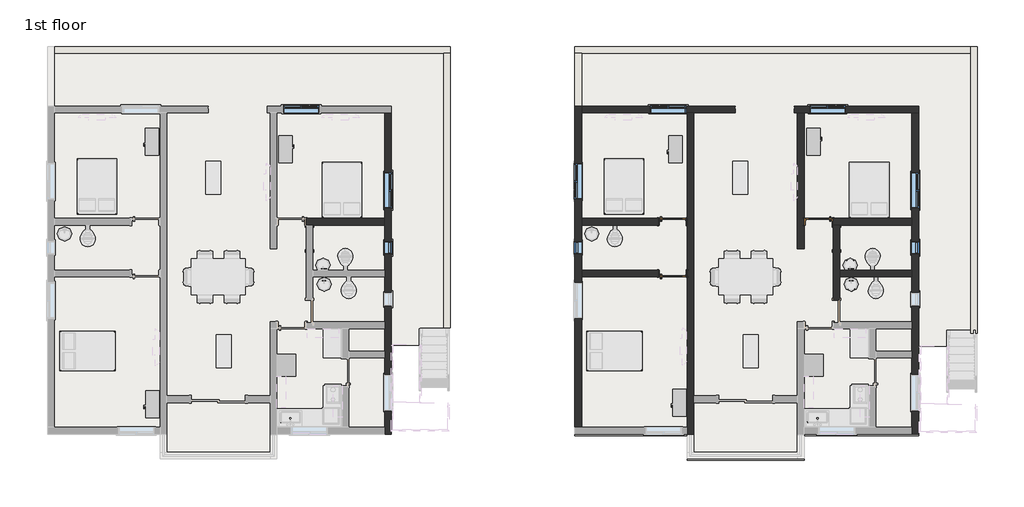
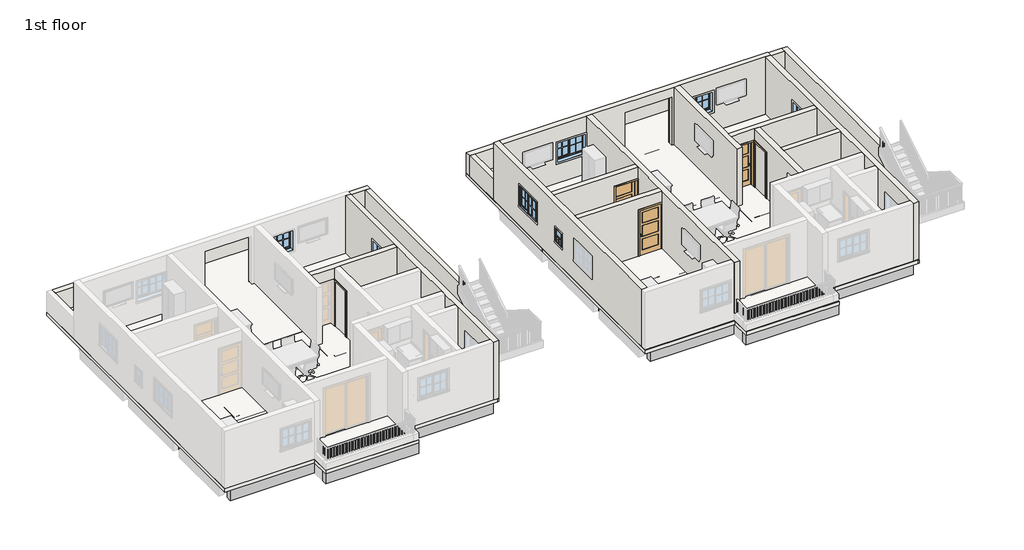
# One storey, part 2 of 8: 18 walls, 14 beams, 9 windows, 5 doors, 2 slabs.
"""IFC4 building model written with IfcOpenShell, lengths in millimetres."""

from ifc_helpers import new_model, si_unit, frame, origin, place, context, project, spatial, polyline, outline, extrude, faceted_brep, transform, mapped, element, save
from components import door_2334f446, door_80766924, door_85036156, window_608ea798, window_2eef0573, window_a5b1ea32

model = new_model("IFC4")

# Units and contexts
model_context = context("Model", 3, world=origin())
ifc_project = project(units=[si_unit("LENGTHUNIT", "METRE", prefix="MILLI")], contexts=[model_context])

# Site, building, storey
site = spatial("IfcSite", under=ifc_project)
building = spatial("IfcBuilding", under=site)
storey = spatial("IfcBuildingStorey", under=building, Name="1st floor", Elevation=3810.0)

# Beams
placement = place(None, origin())
element("IfcBeam", 1, ObjectType="Concrete-Rectangular Beam", at=placement, inside=storey, context=model_context, shape_type="SweptSolid", body=[
    extrude(outline(polyline([(-16071.9993763, -4605.3064015), (-16071.9993763, -4376.7064015), (-12490.5993763, -4376.7064015), (-12490.5993763, -4605.3064015), (-16071.9993763, -4605.3064015)])), frame((0.0, 0.0, 3200.4), z_axis=(0.0, 0.0, 1.0), x_axis=(1.0, 0.0, 0.0)), (0.0, 0.0, 1.0), 609.6),
])
element("IfcBeam", 2, ObjectType="Concrete-Rectangular Beam", at=placement, inside=storey, context=model_context, shape_type="Brep", body=[
    faceted_brep([(-8528.1993763, -5443.5064015, 3810.0), (-8528.1993763, -5214.9064015, 3810.0), (-8756.7993763, -5214.9064015, 3810.0), (-12261.9993763, -5214.9064015, 3810.0), (-12490.5993763, -5214.9064015, 3810.0), (-12490.5993763, -5443.5064015, 3810.0), (-8528.1993763, -5443.5064015, 3200.4), (-12490.5993763, -5443.5064015, 3200.4), (-8528.1993763, -5214.9064015, 3200.4), (-12490.5993763, -5214.9064015, 3200.4), (-12261.9993763, -5214.9064015, 3200.4), (-8756.7993763, -5214.9064015, 3200.4)], [[[0, 1, 2, 3, 4, 5]], [[6, 0, 5, 7]], [[8, 6, 7, 9, 10, 11]], [[1, 8, 11, 10, 9, 4, 3, 2]], [[1, 0, 6, 8]], [[5, 4, 9, 7]]]),
])
element("IfcBeam", 3, ObjectType="Concrete-Rectangular Beam", at=placement, inside=storey, context=model_context, shape_type="Brep", body=[
    faceted_brep([(-8528.1993763, -4376.7064015, 3810.0), (-8528.1993763, -4605.3064015, 3810.0), (-4870.5993763, -4605.3064015, 3810.0), (-4870.5993763, -4376.7064015, 3810.0), (-6089.7993763, -4376.7064015, 3810.0), (-6318.3993763, -4376.7064015, 3810.0), (-8528.1993763, -4376.7064015, 3200.4), (-4870.5993763, -4376.7064015, 3200.4), (-6089.7993763, -4376.7064015, 3200.4), (-6318.3993763, -4376.7064015, 3200.4), (-8528.1993763, -4605.3064015, 3200.4), (-4870.5993763, -4605.3064015, 3200.4)], [[[0, 1, 2, 3, 4, 5]], [[6, 0, 5, 4, 3, 7, 8, 9]], [[10, 6, 9, 8, 7, 11]], [[1, 10, 11, 2]], [[1, 0, 6, 10]], [[3, 2, 11, 7]]]),
])
element("IfcBeam", 4, ObjectType="Concrete-Rectangular Beam", at=placement, inside=storey, context=model_context, shape_type="Brep", body=[
    faceted_brep([(-8528.1993763, -795.3064015, 3810.0), (-8528.1993763, -1023.9064015, 3810.0), (-6318.3993763, -1023.9064015, 3810.0), (-6089.7993763, -1023.9064015, 3810.0), (-4870.5993763, -1023.9064015, 3810.0), (-4870.5993763, -795.3064015, 3810.0), (-7308.9993763, -795.3064015, 3810.0), (-7537.5993763, -795.3064015, 3810.0), (-8528.1993763, -795.3064015, 3200.4), (-4870.5993763, -795.3064015, 3200.4), (-7308.9993763, -795.3064015, 3200.4), (-7537.5993763, -795.3064015, 3200.4), (-8528.1993763, -1023.9064015, 3200.4), (-4870.5993763, -1023.9064015, 3200.4), (-6089.7993763, -1023.9064015, 3200.4), (-6318.3993763, -1023.9064015, 3200.4)], [[[0, 1, 2, 3, 4, 5, 6, 7]], [[8, 0, 7, 6, 5, 9, 10, 11]], [[12, 8, 11, 10, 9, 13, 14, 15]], [[1, 12, 15, 14, 13, 4, 3, 2]], [[1, 0, 8, 12]], [[5, 4, 13, 9]]]),
])
element("IfcBeam", 5, ObjectType="Concrete-Rectangular Beam", at=placement, inside=storey, context=model_context, shape_type="Brep", body=[
    faceted_brep([(-6318.3993763, -4376.7064015, 3810.0), (-6089.7993763, -4376.7064015, 3810.0), (-6089.7993763, -2014.5064015, 3810.0), (-6089.7993763, -1785.9064015, 3810.0), (-6089.7993763, -1023.9064015, 3810.0), (-6318.3993763, -1023.9064015, 3810.0), (-6089.7993763, -4376.7064015, 3200.4), (-6089.7993763, -2014.5064015, 3200.4), (-6089.7993763, -1785.9064015, 3200.4), (-6089.7993763, -1023.9064015, 3200.4), (-6318.3993763, -4376.7064015, 3200.4), (-6318.3993763, -1023.9064015, 3200.4)], [[[0, 1, 2, 3, 4, 5]], [[1, 6, 7, 8, 9, 4, 3, 2]], [[6, 10, 11, 9, 8, 7]], [[10, 0, 5, 11]], [[1, 0, 10, 6]], [[5, 4, 9, 11]]]),
])
element("IfcBeam", 6, ObjectType="Concrete-Rectangular Beam", at=placement, inside=storey, context=model_context, shape_type="SweptSolid", body=[
    extrude(outline(polyline([(-4870.5993763, -1785.9064015), (-4870.5993763, -2014.5064015), (-6089.7993763, -2014.5064015), (-6089.7993763, -1785.9064015), (-4870.5993763, -1785.9064015)])), frame((0.0, 0.0, 3200.4), z_axis=(0.0, 0.0, 1.0), x_axis=(1.0, 0.0, 0.0)), (0.0, 0.0, 1.0), 609.6),
])
element("IfcBeam", 7, ObjectType="Concrete-Rectangular Beam", at=placement, inside=storey, context=model_context, shape_type="Brep", body=[
    faceted_brep([(-8756.7993763, -1023.9064015, 3810.0), (-8756.7993763, -795.3064015, 3810.0), (-12261.9993763, -795.3064015, 3810.0), (-12261.9993763, -1023.9064015, 3810.0), (-8756.7993763, -795.3064015, 3200.4), (-12261.9993763, -795.3064015, 3200.4), (-8756.7993763, -1023.9064015, 3200.4), (-12261.9993763, -1023.9064015, 3200.4)], [[[0, 1, 2, 3]], [[1, 4, 5, 2]], [[4, 6, 7, 5]], [[6, 0, 3, 7]], [[1, 0, 6, 4]], [[3, 2, 5, 7]]]),
    faceted_brep([(-16071.9993763, -1023.9064015, 3810.0), (-16071.9993763, -795.3064015, 3810.0), (-16071.9993763, -795.3064015, 3200.4), (-16071.9993763, -1023.9064015, 3200.4), (-12490.5993763, -795.3064015, 3810.0), (-12490.5993763, -1023.9064015, 3810.0), (-12490.5993763, -1023.9064015, 3200.4), (-12490.5993763, -795.3064015, 3200.4), (-13481.1993763, -795.3064015, 3810.0), (-13709.7993763, -795.3064015, 3810.0), (-13481.1993763, -795.3064015, 3200.4), (-13709.7993763, -795.3064015, 3200.4)], [[[0, 1, 2, 3]], [[4, 5, 6, 7]], [[1, 0, 5, 4, 8, 9]], [[2, 1, 9, 8, 4, 7, 10, 11]], [[3, 2, 11, 10, 7, 6]], [[0, 3, 6, 5]]]),
])
element("IfcBeam", 8, ObjectType="Concrete-Rectangular Beam", at=placement, inside=storey, context=model_context, shape_type="SweptSolid", body=[
    extrude(outline(polyline([(-12261.9993763, -3538.5064015), (-12261.9993763, -3309.9064015), (-8756.7993763, -3309.9064015), (-8756.7993763, -3538.5064015), (-12261.9993763, -3538.5064015)])), frame((0.0, 0.0, 3200.4), z_axis=(0.0, 0.0, 1.0), x_axis=(1.0, 0.0, 0.0)), (0.0, 0.0, 1.0), 609.6),
])
element("IfcBeam", 9, ObjectType="Concrete-Rectangular Beam", at=placement, inside=storey, context=model_context, shape_type="SweptSolid", body=[
    extrude(outline(polyline([(1802.5761273, -4605.3064015), (1802.5761273, -4376.7064015), (5383.9761273, -4376.7064015), (5383.9761273, -4605.3064015), (1802.5761273, -4605.3064015)])), frame((0.0, 0.0, 3200.4), z_axis=(0.0, 0.0, 1.0), x_axis=(1.0, 0.0, 0.0)), (0.0, 0.0, 1.0), 609.6),
])
element("IfcBeam", 10, ObjectType="Concrete-Rectangular Beam", at=placement, inside=storey, context=model_context, shape_type="Brep", body=[
    faceted_brep([(9346.3761273, -5443.5064015, 3810.0), (9346.3761273, -5214.9064015, 3810.0), (9117.7761273, -5214.9064015, 3810.0), (5612.5761273, -5214.9064015, 3810.0), (5383.9761273, -5214.9064015, 3810.0), (5383.9761273, -5443.5064015, 3810.0), (9346.3761273, -5443.5064015, 3200.4), (5383.9761273, -5443.5064015, 3200.4), (9346.3761273, -5214.9064015, 3200.4), (5383.9761273, -5214.9064015, 3200.4), (5612.5761273, -5214.9064015, 3200.4), (9117.7761273, -5214.9064015, 3200.4)], [[[0, 1, 2, 3, 4, 5]], [[6, 0, 5, 7]], [[8, 6, 7, 9, 10, 11]], [[1, 8, 11, 10, 9, 4, 3, 2]], [[1, 0, 6, 8]], [[5, 4, 9, 7]]]),
])
element("IfcBeam", 11, ObjectType="Concrete-Rectangular Beam", at=placement, inside=storey, context=model_context, shape_type="Brep", body=[
    faceted_brep([(9346.3761273, -4376.7064015, 3810.0), (9346.3761273, -4605.3064015, 3810.0), (13003.9761273, -4605.3064015, 3810.0), (13003.9761273, -4376.7064015, 3810.0), (11784.7761273, -4376.7064015, 3810.0), (11556.1761273, -4376.7064015, 3810.0), (9346.3761273, -4376.7064015, 3200.4), (13003.9761273, -4376.7064015, 3200.4), (11784.7761273, -4376.7064015, 3200.4), (11556.1761273, -4376.7064015, 3200.4), (9346.3761273, -4605.3064015, 3200.4), (13003.9761273, -4605.3064015, 3200.4)], [[[0, 1, 2, 3, 4, 5]], [[6, 0, 5, 4, 3, 7, 8, 9]], [[10, 6, 9, 8, 7, 11]], [[1, 10, 11, 2]], [[1, 0, 6, 10]], [[3, 2, 11, 7]]]),
])
element("IfcBeam", 12, ObjectType="Concrete-Rectangular Beam", at=placement, inside=storey, context=model_context, shape_type="Brep", body=[
    faceted_brep([(11556.1761273, -4376.7064015, 3810.0), (11784.7761273, -4376.7064015, 3810.0), (11784.7761273, -2014.5064015, 3810.0), (11784.7761273, -1785.9064015, 3810.0), (11784.7761273, -1023.9064015, 3810.0), (11556.1761273, -1023.9064015, 3810.0), (11784.7761273, -4376.7064015, 3200.4), (11784.7761273, -2014.5064015, 3200.4), (11784.7761273, -1785.9064015, 3200.4), (11784.7761273, -1023.9064015, 3200.4), (11556.1761273, -4376.7064015, 3200.4), (11556.1761273, -1023.9064015, 3200.4)], [[[0, 1, 2, 3, 4, 5]], [[1, 6, 7, 8, 9, 4, 3, 2]], [[6, 10, 11, 9, 8, 7]], [[10, 0, 5, 11]], [[1, 0, 10, 6]], [[5, 4, 9, 11]]]),
])
element("IfcBeam", 13, ObjectType="Concrete-Rectangular Beam", at=placement, inside=storey, context=model_context, shape_type="Brep", body=[
    faceted_brep([(9117.7761273, -1023.9064015, 3810.0), (9117.7761273, -795.3064015, 3810.0), (5612.5761273, -795.3064015, 3810.0), (5612.5761273, -1023.9064015, 3810.0), (9117.7761273, -795.3064015, 3200.4), (5612.5761273, -795.3064015, 3200.4), (9117.7761273, -1023.9064015, 3200.4), (5612.5761273, -1023.9064015, 3200.4)], [[[0, 1, 2, 3]], [[1, 4, 5, 2]], [[4, 6, 7, 5]], [[6, 0, 3, 7]], [[1, 0, 6, 4]], [[3, 2, 5, 7]]]),
    faceted_brep([(1802.5761273, -1023.9064015, 3810.0), (1802.5761273, -795.3064015, 3810.0), (1802.5761273, -795.3064015, 3200.4), (1802.5761273, -1023.9064015, 3200.4), (5383.9761273, -795.3064015, 3810.0), (5383.9761273, -1023.9064015, 3810.0), (5383.9761273, -1023.9064015, 3200.4), (5383.9761273, -795.3064015, 3200.4), (4393.3761273, -795.3064015, 3810.0), (4164.7761273, -795.3064015, 3810.0), (4393.3761273, -795.3064015, 3200.4), (4164.7761273, -795.3064015, 3200.4)], [[[0, 1, 2, 3]], [[4, 5, 6, 7]], [[1, 0, 5, 4, 8, 9]], [[2, 1, 9, 8, 4, 7, 10, 11]], [[3, 2, 11, 10, 7, 6]], [[0, 3, 6, 5]]]),
])
element("IfcBeam", 14, ObjectType="Concrete-Rectangular Beam", at=placement, inside=storey, context=model_context, shape_type="SweptSolid", body=[
    extrude(outline(polyline([(5612.5761273, -3538.5064015), (5612.5761273, -3309.9064015), (9117.7761273, -3309.9064015), (9117.7761273, -3538.5064015), (5612.5761273, -3538.5064015)])), frame((0.0, 0.0, 3200.4), z_axis=(0.0, 0.0, 1.0), x_axis=(1.0, 0.0, 0.0)), (0.0, 0.0, 1.0), 609.6),
])

# Doors
door_shape = door_2334f446(model_context)
element("IfcDoor", 15, ObjectType="Door-Interior-Single-3_Panel_Vert-Wood : 36\" x 80\"", at=placement, inside=storey, context=model_context, shape_type="MappedRepresentation", body=[
    mapped(door_shape, transform((4888.6761273, 2598.7685985, 3810.0), x_axis=(1.0, 0.0, 0.0), y_axis=(0.0, 1.0, 0.0), z_axis=(0.0, 0.0, 1.0))),
])
door_2_shape = door_80766924(model_context)
element("IfcDoor", 16, ObjectType="Door-Interior-Single-3_Panel_Vert-Wood : 36\" x 80\"", at=placement, inside=storey, context=model_context, shape_type="MappedRepresentation", body=[
    mapped(door_2_shape, transform((4888.6761273, 839.8185985, 3810.0), x_axis=(1.0, 0.0, 0.0), y_axis=(0.0, 1.0, 0.0), z_axis=(0.0, 0.0, 1.0))),
])
element("IfcDoor", 17, ObjectType="Door-Interior-Single-3_Panel_Vert-Wood : 36\" x 80\"", at=placement, inside=storey, context=model_context, shape_type="MappedRepresentation", body=[
    mapped(door_2_shape, transform((9841.6761273, 2598.7685985, 3810.0), x_axis=(-1.0, 0.0, 0.0), y_axis=(0.0, -1.0, 0.0), z_axis=(0.0, 0.0, 1.0))),
])
door_3_shape = door_85036156(model_context)
element("IfcDoor", 18, ObjectType="Single-Flush : 30\" x 80\"", at=placement, inside=storey, context=model_context, shape_type="MappedRepresentation", body=[
    mapped(door_3_shape, transform((-7423.2993763, 2024.0935985, 3810.0), x_axis=(0.0, 1.0, 0.0), y_axis=(-1.0, 0.0, 0.0), z_axis=(0.0, 0.0, 1.0))),
])
element("IfcDoor", 19, ObjectType="Single-Flush : 30\" x 80\"", at=placement, inside=storey, context=model_context, shape_type="MappedRepresentation", body=[
    mapped(door_3_shape, transform((10451.2761273, 2024.0935985, 3810.0), x_axis=(0.0, 1.0, 0.0), y_axis=(-1.0, 0.0, 0.0), z_axis=(0.0, 0.0, 1.0))),
])

# Slabs
element("IfcSlab", 20, at=placement, inside=storey, context=model_context, shape_type="SweptSolid", body=[
    extrude(outline(polyline([(-2647.3594779, 8539.1935985), (-2647.3594779, -998.5064015), (-3676.7993763, -998.5064015), (-3676.7993763, -1582.7064015), (-4641.9993763, -1582.7064015), (-4641.9993763, -4605.3064015), (-4692.7993763, -4605.3064015), (-8528.1993763, -4605.3064015), (-8528.1993763, -5443.5064015), (-12490.5993763, -5443.5064015), (-12490.5993763, -4611.6564015), (-16300.5993763, -4611.6564015), (-16300.5993763, 8539.1935985), (-2647.3594779, 8539.1935985)])), frame((0.0, 0.0, 3657.6), z_axis=(0.0, 0.0, 1.0), x_axis=(1.0, 0.0, 0.0)), (0.0, 0.0, 1.0), 152.4),
])
element("IfcSlab", 21, at=placement, inside=storey, context=model_context, shape_type="SweptSolid", body=[
    extrude(outline(polyline([(15227.2160257, 8539.1935985), (15227.2160257, -1093.7564015), (14197.7761273, -1093.7564015), (14197.7761273, -1627.1564015), (13232.5761273, -1627.1564015), (13232.5761273, -4649.7564015), (13181.7761273, -4649.7564015), (9346.3761273, -4649.7564015), (9346.3761273, -5487.9564015), (5383.9761273, -5487.9564015), (5383.9761273, -4656.1064015), (1573.9761273, -4656.1064015), (1573.9761273, 8539.1935985), (15227.2160257, 8539.1935985)])), frame((0.0, 0.0, 3657.6), z_axis=(0.0, 0.0, 1.0), x_axis=(1.0, 0.0, 0.0)), (0.0, 0.0, 1.0), 152.4),
])

# Walls
element("IfcWall", 22, at=placement, inside=storey, context=model_context, shape_type="Brep", body=[
    faceted_brep([(-4870.5993763, 6291.2935985, 3810.0), (-4870.5993763, 2709.8935985, 3810.0), (-4870.5993763, 2481.2935985, 3810.0), (-4870.5993763, 957.2935985, 3810.0), (-4870.5993763, 728.6935985, 3810.0), (-4870.5993763, -795.3064015, 3810.0), (-4870.5993763, -1023.9064015, 3810.0), (-4870.5993763, -1785.9064015, 3810.0), (-4870.5993763, -2014.5064015, 3810.0), (-4870.5993763, -4376.7064015, 3810.0), (-4870.5993763, -4605.3064015, 3810.0), (-4870.5993763, -4605.3064015, 6400.8), (-4870.5993763, -4376.7064015, 6400.8), (-4870.5993763, -2014.5064015, 6400.8), (-4870.5993763, -1785.9064015, 6400.8), (-4870.5993763, -1023.9064015, 6400.8), (-4870.5993763, -795.3064015, 6400.8), (-4870.5993763, 728.6935985, 6400.8), (-4870.5993763, 957.2935985, 6400.8), (-4870.5993763, 2481.2935985, 6400.8), (-4870.5993763, 2709.8935985, 6400.8), (-4870.5993763, 6291.2935985, 6400.8), (-4870.5993763, 4271.9935985, 5638.8), (-4870.5993763, 3052.7935985, 5638.8), (-4870.5993763, 3052.7935985, 4724.4), (-4870.5993763, 4271.9935985, 4724.4), (-4870.5993763, -249.2064015, 5334.0), (-4870.5993763, -249.2064015, 4724.4), (-4870.5993763, 182.5935985, 4724.4), (-4870.5993763, 182.5935985, 5334.0), (-4870.5993763, 1503.3935985, 5334.0), (-4870.5993763, 1503.3935985, 4724.4), (-4870.5993763, 1935.1935985, 4724.4), (-4870.5993763, 1935.1935985, 5334.0), (-4870.5993763, -3805.2064015, 5638.8), (-4870.5993763, -3805.2064015, 4724.4), (-4870.5993763, -2586.0064015, 4724.4), (-4870.5993763, -2586.0064015, 5638.8), (-4641.9993763, 6291.2935985, 3810.0), (-4641.9993763, 6291.2935985, 6400.8), (-4641.9993763, -4605.3064015, 6400.8), (-4641.9993763, -4605.3064015, 3810.0), (-4641.9993763, 4271.9935985, 5638.8), (-4641.9993763, 4271.9935985, 4724.4), (-4641.9993763, 3052.7935985, 4724.4), (-4641.9993763, 3052.7935985, 5638.8), (-4641.9993763, -249.2064015, 5334.0), (-4641.9993763, 182.5935985, 5334.0), (-4641.9993763, 182.5935985, 4724.4), (-4641.9993763, -249.2064015, 4724.4), (-4641.9993763, 1503.3935985, 5334.0), (-4641.9993763, 1935.1935985, 5334.0), (-4641.9993763, 1935.1935985, 4724.4), (-4641.9993763, 1503.3935985, 4724.4), (-4641.9993763, -3805.2064015, 5638.8), (-4641.9993763, -2586.0064015, 5638.8), (-4641.9993763, -2586.0064015, 4724.4), (-4641.9993763, -3805.2064015, 4724.4)], [[[0, 1, 2, 3, 4, 5, 6, 7, 8, 9, 10, 11, 12, 13, 14, 15, 16, 17, 18, 19, 20, 21], [22, 23, 24, 25], [26, 27, 28, 29], [30, 31, 32, 33], [34, 35, 36, 37]], [[38, 39, 40, 41], [42, 43, 44, 45], [46, 47, 48, 49], [50, 51, 52, 53], [54, 55, 56, 57]], [[10, 9, 8, 7, 6, 5, 4, 3, 2, 1, 0, 38, 41]], [[21, 20, 19, 18, 17, 16, 15, 14, 13, 12, 11, 40, 39]], [[0, 21, 39, 38]], [[11, 10, 41, 40]], [[43, 42, 22, 25]], [[44, 43, 25, 24]], [[45, 44, 24, 23]], [[42, 45, 23, 22]], [[27, 26, 46, 49]], [[28, 27, 49, 48]], [[29, 28, 48, 47]], [[26, 29, 47, 46]], [[31, 30, 50, 53]], [[32, 31, 53, 52]], [[33, 32, 52, 51]], [[30, 33, 51, 50]], [[35, 34, 54, 57]], [[36, 35, 57, 56]], [[37, 36, 56, 55]], [[34, 37, 55, 54]]]),
])
element("IfcWall", 23, at=placement, inside=storey, context=model_context, shape_type="Brep", body=[
    faceted_brep([(-4870.5993763, 2481.2935985, 6400.8), (-7308.9993763, 2481.2935985, 6400.8), (-7537.5993763, 2481.2935985, 6400.8), (-8528.1993763, 2481.2935985, 6400.8), (-8528.1993763, 2481.2935985, 3810.0), (-8515.4993763, 2481.2935985, 3810.0), (-8515.4993763, 2481.2935985, 5867.4), (-7550.2993763, 2481.2935985, 5867.4), (-7550.2993763, 2481.2935985, 3810.0), (-7537.5993763, 2481.2935985, 3810.0), (-7308.9993763, 2481.2935985, 3810.0), (-4870.5993763, 2481.2935985, 3810.0), (-8528.1993763, 2709.8935985, 6400.8), (-4870.5993763, 2709.8935985, 6400.8), (-4870.5993763, 2709.8935985, 3810.0), (-7550.2993763, 2709.8935985, 3810.0), (-7550.2993763, 2709.8935985, 5867.4), (-8515.4993763, 2709.8935985, 5867.4), (-8515.4993763, 2709.8935985, 3810.0), (-8528.1993763, 2709.8935985, 3810.0)], [[[0, 1, 2, 3, 4, 5, 6, 7, 8, 9, 10, 11]], [[12, 13, 14, 15, 16, 17, 18, 19]], [[14, 11, 10, 9, 8, 15]], [[4, 19, 18, 5]], [[3, 2, 1, 0, 13, 12]], [[0, 11, 14, 13]], [[17, 6, 5, 18]], [[6, 17, 16, 7]], [[7, 16, 15, 8]], [[4, 3, 12, 19]]]),
])
element("IfcWall", 24, at=placement, inside=storey, context=model_context, shape_type="Brep", body=[
    faceted_brep([(1573.9761273, 6519.8935985, 3810.0), (1573.9761273, -4376.7064015, 3810.0), (1573.9761273, -4376.7064015, 6400.8), (1573.9761273, 6519.8935985, 6400.8), (1573.9761273, 4576.7935985, 5638.8), (1573.9761273, 3357.5935985, 5638.8), (1573.9761273, 3357.5935985, 4724.4), (1573.9761273, 4576.7935985, 4724.4), (1573.9761273, -681.0064015, 5638.8), (1573.9761273, -681.0064015, 4724.4), (1573.9761273, 538.1935985, 4724.4), (1573.9761273, 538.1935985, 5638.8), (1573.9761273, 1935.1935985, 5334.0), (1573.9761273, 1503.3935985, 5334.0), (1573.9761273, 1503.3935985, 4724.4), (1573.9761273, 1935.1935985, 4724.4), (1802.5761273, 6519.8935985, 3810.0), (1802.5761273, 6519.8935985, 6400.8), (1802.5761273, 6291.2935985, 6400.8), (1802.5761273, 2709.8935985, 6400.8), (1802.5761273, 2481.2935985, 6400.8), (1802.5761273, 957.2935985, 6400.8), (1802.5761273, 728.6935985, 6400.8), (1802.5761273, -4376.7064015, 6400.8), (1802.5761273, -4376.7064015, 3810.0), (1802.5761273, 728.6935985, 3810.0), (1802.5761273, 957.2935985, 3810.0), (1802.5761273, 2481.2935985, 3810.0), (1802.5761273, 2709.8935985, 3810.0), (1802.5761273, 6291.2935985, 3810.0), (1802.5761273, 4576.7935985, 5638.8), (1802.5761273, 4576.7935985, 4724.4), (1802.5761273, 3357.5935985, 4724.4), (1802.5761273, 3357.5935985, 5638.8), (1802.5761273, -681.0064015, 5638.8), (1802.5761273, 538.1935985, 5638.8), (1802.5761273, 538.1935985, 4724.4), (1802.5761273, -681.0064015, 4724.4), (1802.5761273, 1935.1935985, 5334.0), (1802.5761273, 1935.1935985, 4724.4), (1802.5761273, 1503.3935985, 4724.4), (1802.5761273, 1503.3935985, 5334.0)], [[[0, 1, 2, 3], [4, 5, 6, 7], [8, 9, 10, 11], [12, 13, 14, 15]], [[16, 17, 18, 19, 20, 21, 22, 23, 24, 25, 26, 27, 28, 29], [30, 31, 32, 33], [34, 35, 36, 37], [38, 39, 40, 41]], [[1, 0, 16, 29, 28, 27, 26, 25, 24]], [[3, 2, 23, 22, 21, 20, 19, 18, 17]], [[0, 3, 17, 16]], [[2, 1, 24, 23]], [[31, 30, 4, 7]], [[32, 31, 7, 6]], [[33, 32, 6, 5]], [[30, 33, 5, 4]], [[9, 8, 34, 37]], [[10, 9, 37, 36]], [[11, 10, 36, 35]], [[8, 11, 35, 34]], [[39, 38, 12, 15]], [[40, 39, 15, 14]], [[41, 40, 14, 13]], [[38, 41, 13, 12]]]),
])
element("IfcWall", 25, at=placement, inside=storey, context=model_context, shape_type="SweptSolid", body=[
    extrude(outline(polyline([(6400.8, 5383.9761273), (6400.8, 1802.5761273), (3810.0, 1802.5761273), (3810.0, 4406.0761273), (5867.4, 4406.0761273), (5867.4, 5371.2761273), (3810.0, 5371.2761273), (3810.0, 5383.9761273), (6400.8, 5383.9761273)])), frame((0.0, 2481.2935985, 0.0), z_axis=(0.0, 1.0, 0.0), x_axis=(0.0, 0.0, 1.0)), (0.0, 0.0, 1.0), 228.6),
])
element("IfcWall", 26, at=placement, inside=storey, context=model_context, shape_type="Brep", body=[
    faceted_brep([(13232.5761273, 6291.2935985, 6400.8), (13003.9761273, 6291.2935985, 6400.8), (9346.3761273, 6291.2935985, 6400.8), (9117.7761273, 6291.2935985, 6400.8), (5612.5761273, 6291.2935985, 6400.8), (5383.9761273, 6291.2935985, 6400.8), (1802.5761273, 6291.2935985, 6400.8), (1802.5761273, 6291.2935985, 3810.0), (5383.9761273, 6291.2935985, 3810.0), (5612.5761273, 6291.2935985, 3810.0), (7012.8761273, 6291.2935985, 3810.0), (7012.8761273, 6291.2935985, 5979.5), (9012.8761273, 6291.2935985, 5979.5), (9012.8761273, 6291.2935985, 3810.0), (9117.7761273, 6291.2935985, 3810.0), (9346.3761273, 6291.2935985, 3810.0), (13003.9761273, 6291.2935985, 3810.0), (13232.5761273, 6291.2935985, 3810.0), (9536.8761273, 6291.2935985, 5638.8), (10756.0761273, 6291.2935985, 5638.8), (10756.0761273, 6291.2935985, 4724.4), (9536.8761273, 6291.2935985, 4724.4), (5345.8761273, 6291.2935985, 5638.8), (5345.8761273, 6291.2935985, 4724.4), (4126.6761273, 6291.2935985, 4724.4), (4126.6761273, 6291.2935985, 5638.8), (1802.5761273, 6519.8935985, 6400.8), (13232.5761273, 6519.8935985, 6400.8), (13232.5761273, 6519.8935985, 3810.0), (9012.8761273, 6519.8935985, 3810.0), (9012.8761273, 6519.8935985, 5979.5), (7012.8761273, 6519.8935985, 5979.5), (7012.8761273, 6519.8935985, 3810.0), (1802.5761273, 6519.8935985, 3810.0), (9536.8761273, 6519.8935985, 5638.8), (9536.8761273, 6519.8935985, 4724.4), (10756.0761273, 6519.8935985, 4724.4), (10756.0761273, 6519.8935985, 5638.8), (5345.8761273, 6519.8935985, 5638.8), (4126.6761273, 6519.8935985, 5638.8), (4126.6761273, 6519.8935985, 4724.4), (5345.8761273, 6519.8935985, 4724.4), (7012.8761273, 6499.8935985, 3810.0), (6997.8761273, 6499.8935985, 3810.0), (6997.8761273, 6429.8935985, 3810.0), (7012.8761273, 6429.8935985, 3810.0), (9012.8761273, 6429.8935985, 3810.0), (9027.8761273, 6429.8935985, 3810.0), (9027.8761273, 6499.8935985, 3810.0), (9012.8761273, 6499.8935985, 3810.0), (9012.8761273, 6499.8935985, 5979.5), (7012.8761273, 6499.8935985, 5979.5), (7012.8761273, 6429.8935985, 5979.5), (9012.8761273, 6429.8935985, 5979.5), (6997.8761273, 6429.8935985, 5994.5), (9027.8761273, 6429.8935985, 5994.5), (9027.8761273, 6499.8935985, 5994.5), (6997.8761273, 6499.8935985, 5994.5)], [[[0, 1, 2, 3, 4, 5, 6, 7, 8, 9, 10, 11, 12, 13, 14, 15, 16, 17], [18, 19, 20, 21], [22, 23, 24, 25]], [[26, 27, 28, 29, 30, 31, 32, 33], [34, 35, 36, 37], [38, 39, 40, 41]], [[7, 33, 32, 42, 43, 44, 45, 10, 9, 8]], [[28, 17, 16, 15, 14, 13, 46, 47, 48, 49, 29]], [[6, 5, 4, 3, 2, 1, 0, 27, 26]], [[7, 6, 26, 33]], [[0, 17, 28, 27]], [[50, 51, 31, 30]], [[52, 53, 12, 11]], [[45, 52, 11, 10]], [[53, 46, 13, 12]], [[53, 52, 45, 44, 54, 55, 47, 46]], [[47, 55, 56, 48]], [[51, 50, 49, 48, 56, 57, 43, 42]], [[49, 50, 30, 29]], [[51, 42, 32, 31]], [[54, 44, 43, 57]], [[55, 54, 57, 56]], [[35, 34, 18, 21]], [[36, 35, 21, 20]], [[37, 36, 20, 19]], [[34, 37, 19, 18]], [[23, 22, 38, 41]], [[24, 23, 41, 40]], [[25, 24, 40, 39]], [[22, 25, 39, 38]]]),
])
element("IfcWall", 27, at=placement, inside=storey, context=model_context, shape_type="Brep", body=[
    faceted_brep([(13003.9761273, 6291.2935985, 3810.0), (13003.9761273, 2709.8935985, 3810.0), (13003.9761273, 2481.2935985, 3810.0), (13003.9761273, 957.2935985, 3810.0), (13003.9761273, 728.6935985, 3810.0), (13003.9761273, -795.3064015, 3810.0), (13003.9761273, -1023.9064015, 3810.0), (13003.9761273, -1785.9064015, 3810.0), (13003.9761273, -2014.5064015, 3810.0), (13003.9761273, -4376.7064015, 3810.0), (13003.9761273, -4605.3064015, 3810.0), (13003.9761273, -4605.3064015, 6400.8), (13003.9761273, -4376.7064015, 6400.8), (13003.9761273, -2014.5064015, 6400.8), (13003.9761273, -1785.9064015, 6400.8), (13003.9761273, -1023.9064015, 6400.8), (13003.9761273, -795.3064015, 6400.8), (13003.9761273, 728.6935985, 6400.8), (13003.9761273, 957.2935985, 6400.8), (13003.9761273, 2481.2935985, 6400.8), (13003.9761273, 2709.8935985, 6400.8), (13003.9761273, 6291.2935985, 6400.8), (13003.9761273, 4271.9935985, 5638.8), (13003.9761273, 3052.7935985, 5638.8), (13003.9761273, 3052.7935985, 4724.4), (13003.9761273, 4271.9935985, 4724.4), (13003.9761273, -249.2064015, 5334.0), (13003.9761273, -249.2064015, 4724.4), (13003.9761273, 182.5935985, 4724.4), (13003.9761273, 182.5935985, 5334.0), (13003.9761273, 1503.3935985, 5334.0), (13003.9761273, 1503.3935985, 4724.4), (13003.9761273, 1935.1935985, 4724.4), (13003.9761273, 1935.1935985, 5334.0), (13003.9761273, -3805.2064015, 5638.8), (13003.9761273, -3805.2064015, 4724.4), (13003.9761273, -2586.0064015, 4724.4), (13003.9761273, -2586.0064015, 5638.8), (13232.5761273, 6291.2935985, 3810.0), (13232.5761273, 6291.2935985, 6400.8), (13232.5761273, -4605.3064015, 6400.8), (13232.5761273, -4605.3064015, 3810.0), (13232.5761273, 4271.9935985, 5638.8), (13232.5761273, 4271.9935985, 4724.4), (13232.5761273, 3052.7935985, 4724.4), (13232.5761273, 3052.7935985, 5638.8), (13232.5761273, -249.2064015, 5334.0), (13232.5761273, 182.5935985, 5334.0), (13232.5761273, 182.5935985, 4724.4), (13232.5761273, -249.2064015, 4724.4), (13232.5761273, 1503.3935985, 5334.0), (13232.5761273, 1935.1935985, 5334.0), (13232.5761273, 1935.1935985, 4724.4), (13232.5761273, 1503.3935985, 4724.4), (13232.5761273, -3805.2064015, 5638.8), (13232.5761273, -2586.0064015, 5638.8), (13232.5761273, -2586.0064015, 4724.4), (13232.5761273, -3805.2064015, 4724.4)], [[[0, 1, 2, 3, 4, 5, 6, 7, 8, 9, 10, 11, 12, 13, 14, 15, 16, 17, 18, 19, 20, 21], [22, 23, 24, 25], [26, 27, 28, 29], [30, 31, 32, 33], [34, 35, 36, 37]], [[38, 39, 40, 41], [42, 43, 44, 45], [46, 47, 48, 49], [50, 51, 52, 53], [54, 55, 56, 57]], [[10, 9, 8, 7, 6, 5, 4, 3, 2, 1, 0, 38, 41]], [[21, 20, 19, 18, 17, 16, 15, 14, 13, 12, 11, 40, 39]], [[0, 21, 39, 38]], [[11, 10, 41, 40]], [[43, 42, 22, 25]], [[44, 43, 25, 24]], [[45, 44, 24, 23]], [[42, 45, 23, 22]], [[27, 26, 46, 49]], [[28, 27, 49, 48]], [[29, 28, 48, 47]], [[26, 29, 47, 46]], [[31, 30, 50, 53]], [[32, 31, 53, 52]], [[33, 32, 52, 51]], [[30, 33, 51, 50]], [[35, 34, 54, 57]], [[36, 35, 57, 56]], [[37, 36, 56, 55]], [[34, 37, 55, 54]]]),
])
element("IfcWall", 28, at=placement, inside=storey, context=model_context, shape_type="Brep", body=[
    faceted_brep([(9117.7761273, 6291.2935985, 3810.0), (9117.7761273, 1681.1935985, 3810.0), (9117.7761273, 1681.1935985, 6400.8), (9117.7761273, 6291.2935985, 6400.8), (9346.3761273, 6291.2935985, 3810.0), (9346.3761273, 6291.2935985, 6400.8), (9346.3761273, 2709.8935985, 6400.8), (9346.3761273, 2481.2935985, 6400.8), (9346.3761273, 1681.1935985, 6400.8), (9346.3761273, 1681.1935985, 3810.0), (9346.3761273, 2481.2935985, 3810.0), (9346.3761273, 2709.8935985, 3810.0)], [[[0, 1, 2, 3]], [[4, 5, 6, 7, 8, 9, 10, 11]], [[1, 0, 4, 11, 10, 9]], [[2, 1, 9, 8]], [[3, 2, 8, 7, 6, 5]], [[0, 3, 5, 4]]]),
])
element("IfcWall", 29, at=placement, inside=storey, context=model_context, shape_type="SweptSolid", body=[
    extrude(outline(polyline([(10565.5761273, 957.2935985), (13003.9761273, 957.2935985), (13003.9761273, 728.6935985), (10565.5761273, 728.6935985), (10565.5761273, 957.2935985)])), frame((0.0, 0.0, 3810.0), z_axis=(0.0, 0.0, 1.0), x_axis=(1.0, 0.0, 0.0)), (0.0, 0.0, 1.0), 2590.8),
])
element("IfcWall", 30, at=placement, inside=storey, context=model_context, shape_type="Brep", body=[
    faceted_brep([(10565.5761273, 2481.2935985, 6400.8), (10565.5761273, 957.2935985, 6400.8), (10565.5761273, 728.6935985, 6400.8), (10565.5761273, -795.3064015, 6400.8), (10565.5761273, -795.3064015, 5842.0), (10565.5761273, -71.4064015, 5842.0), (10565.5761273, -71.4064015, 3810.0), (10565.5761273, 728.6935985, 3810.0), (10565.5761273, 957.2935985, 3810.0), (10565.5761273, 2481.2935985, 3810.0), (10336.9761273, -795.3064015, 6400.8), (10336.9761273, 2481.2935985, 6400.8), (10336.9761273, 2481.2935985, 3810.0), (10336.9761273, -71.4064015, 3810.0), (10336.9761273, -71.4064015, 5842.0), (10336.9761273, -795.3064015, 5842.0)], [[[0, 1, 2, 3, 4, 5, 6, 7, 8, 9]], [[10, 11, 12, 13, 14, 15]], [[12, 9, 8, 7, 6, 13]], [[3, 2, 1, 0, 11, 10]], [[3, 10, 15, 4]], [[0, 9, 12, 11]], [[14, 5, 4, 15]], [[5, 14, 13, 6]]]),
])
element("IfcWall", 31, at=placement, inside=storey, context=model_context, shape_type="SweptSolid", body=[
    extrude(outline(polyline([(2481.2935985, 3810.0), (2405.0935985, 3810.0), (2405.0935985, 5842.0), (1643.0935985, 5842.0), (1643.0935985, 3810.0), (957.2935985, 3810.0), (957.2935985, 6400.8), (2481.2935985, 6400.8), (2481.2935985, 3810.0)])), frame((10336.9761273, 0.0, 0.0), z_axis=(1.0, 0.0, 0.0), x_axis=(0.0, 1.0, 0.0)), (0.0, 0.0, 1.0), 228.6),
])
element("IfcWall", 32, at=placement, inside=storey, context=model_context, shape_type="Brep", body=[
    faceted_brep([(13003.9761273, 2481.2935985, 6400.8), (10565.5761273, 2481.2935985, 6400.8), (10336.9761273, 2481.2935985, 6400.8), (9346.3761273, 2481.2935985, 6400.8), (9346.3761273, 2481.2935985, 3810.0), (9359.0761273, 2481.2935985, 3810.0), (9359.0761273, 2481.2935985, 5867.4), (10324.2761273, 2481.2935985, 5867.4), (10324.2761273, 2481.2935985, 3810.0), (10336.9761273, 2481.2935985, 3810.0), (10565.5761273, 2481.2935985, 3810.0), (13003.9761273, 2481.2935985, 3810.0), (9346.3761273, 2709.8935985, 6400.8), (13003.9761273, 2709.8935985, 6400.8), (13003.9761273, 2709.8935985, 3810.0), (10324.2761273, 2709.8935985, 3810.0), (10324.2761273, 2709.8935985, 5867.4), (9359.0761273, 2709.8935985, 5867.4), (9359.0761273, 2709.8935985, 3810.0), (9346.3761273, 2709.8935985, 3810.0)], [[[0, 1, 2, 3, 4, 5, 6, 7, 8, 9, 10, 11]], [[12, 13, 14, 15, 16, 17, 18, 19]], [[14, 11, 10, 9, 8, 15]], [[4, 19, 18, 5]], [[3, 2, 1, 0, 13, 12]], [[0, 11, 14, 13]], [[17, 6, 5, 18]], [[6, 17, 16, 7]], [[7, 16, 15, 8]], [[4, 3, 12, 19]]]),
])
element("IfcWall", 33, at=placement, inside=storey, context=model_context, shape_type="SweptSolid", body=[
    extrude(outline(polyline([(6400.8, 5383.9761273), (6400.8, 1802.5761273), (3810.0, 1802.5761273), (3810.0, 4406.0761273), (5867.4, 4406.0761273), (5867.4, 5371.2761273), (3810.0, 5371.2761273), (3810.0, 5383.9761273), (6400.8, 5383.9761273)])), frame((0.0, 728.6935985, 0.0), z_axis=(0.0, 1.0, 0.0), x_axis=(0.0, 0.0, 1.0)), (0.0, 0.0, 1.0), 228.6),
])
element("IfcWall", 34, at=placement, inside=storey, context=model_context, shape_type="Brep", body=[
    faceted_brep([(5612.5761273, -4605.3064015, 3810.0), (5612.5761273, -3538.5064015, 3810.0), (5612.5761273, -3309.9064015, 3810.0), (5612.5761273, 6291.2935985, 3810.0), (5612.5761273, 6291.2935985, 6400.8), (5612.5761273, -3309.9064015, 6400.8), (5612.5761273, -3538.5064015, 6400.8), (5612.5761273, -4605.3064015, 6400.8), (5383.9761273, -4605.3064015, 3810.0), (5383.9761273, -4605.3064015, 6400.8), (5383.9761273, -4376.7064015, 6400.8), (5383.9761273, 728.6935985, 6400.8), (5383.9761273, 957.2935985, 6400.8), (5383.9761273, 2481.2935985, 6400.8), (5383.9761273, 2709.8935985, 6400.8), (5383.9761273, 6291.2935985, 6400.8), (5383.9761273, 6291.2935985, 3810.0), (5383.9761273, 2709.8935985, 3810.0), (5383.9761273, 2481.2935985, 3810.0), (5383.9761273, 957.2935985, 3810.0), (5383.9761273, 728.6935985, 3810.0), (5383.9761273, -4376.7064015, 3810.0)], [[[0, 1, 2, 3, 4, 5, 6, 7]], [[8, 9, 10, 11, 12, 13, 14, 15, 16, 17, 18, 19, 20, 21]], [[3, 2, 1, 0, 8, 21, 20, 19, 18, 17, 16]], [[7, 6, 5, 4, 15, 14, 13, 12, 11, 10, 9]], [[4, 3, 16, 15]], [[0, 7, 9, 8]]]),
])
element("IfcWall", 35, at=placement, inside=storey, context=model_context, shape_type="Brep", body=[
    faceted_brep([(15227.2160257, -1179.4814015, 3810.0), (15227.2160257, 8539.1935985, 3810.0), (15227.2160257, 8539.1935985, 4724.4), (15227.2160257, -1179.4814015, 4724.4), (14998.6160257, -1179.4814015, 3810.0), (14998.6160257, -1179.4814015, 4724.4), (14998.6160257, 8310.5935985, 4724.4), (14998.6160257, 8539.1935985, 4724.4), (14998.6160257, 8539.1935985, 3810.0), (14998.6160257, 8310.5935985, 3810.0)], [[[0, 1, 2, 3]], [[4, 5, 6, 7, 8, 9]], [[1, 0, 4, 9, 8]], [[3, 2, 7, 6, 5]], [[0, 3, 5, 4]], [[2, 1, 8, 7]]]),
])
element("IfcWall", 36, at=placement, inside=storey, context=model_context, shape_type="Brep", body=[
    faceted_brep([(14998.6160257, 8539.1935985, 3810.0), (1573.9761273, 8539.1935985, 3810.0), (1573.9761273, 8539.1935985, 4724.4), (14998.6160257, 8539.1935985, 4724.4), (14998.6160257, 8310.5935985, 3810.0), (14998.6160257, 8310.5935985, 4724.4), (1802.5761273, 8310.5935985, 4724.4), (1573.9761273, 8310.5935985, 4724.4), (1573.9761273, 8310.5935985, 3810.0), (1802.5761273, 8310.5935985, 3810.0)], [[[0, 1, 2, 3]], [[4, 5, 6, 7, 8, 9]], [[1, 0, 4, 9, 8]], [[3, 2, 7, 6, 5]], [[0, 3, 5, 4]], [[2, 1, 8, 7]]]),
])
element("IfcWall", 37, at=placement, inside=storey, context=model_context, shape_type="SweptSolid", body=[
    extrude(outline(polyline([(1573.9761273, 6275.4185985), (1573.9761273, 8310.5935985), (1802.5761273, 8310.5935985), (1802.5761273, 6275.4185985), (1573.9761273, 6275.4185985)])), frame((0.0, 0.0, 3810.0), z_axis=(0.0, 0.0, 1.0), x_axis=(1.0, 0.0, 0.0)), (0.0, 0.0, 1.0), 914.4),
])
element("IfcWall", 38, at=placement, inside=storey, context=model_context, shape_type="Brep", body=[
    faceted_brep([(-16071.9993763, 8310.5935985, 3810.0), (-2875.9594779, 8310.5935985, 3810.0), (-2647.3594779, 8310.5935985, 3810.0), (-2647.3594779, 8310.5935985, 4724.4), (-2875.9594779, 8310.5935985, 4724.4), (-16071.9993763, 8310.5935985, 4724.4), (-16071.9993763, 8539.1935985, 3810.0), (-16071.9993763, 8539.1935985, 4724.4), (-2647.3594779, 8539.1935985, 4724.4), (-2647.3594779, 8539.1935985, 3810.0)], [[[0, 1, 2, 3, 4, 5]], [[6, 7, 8, 9]], [[2, 1, 0, 6, 9]], [[5, 4, 3, 8, 7]], [[0, 5, 7, 6]], [[3, 2, 9, 8]]]),
])
element("IfcWall", 39, at=placement, inside=storey, context=model_context, shape_type="SweptSolid", body=[
    extrude(outline(polyline([(-2875.9594779, -998.5064015), (-2875.9594779, 8310.5935985), (-2647.3594779, 8310.5935985), (-2647.3594779, -998.5064015), (-2875.9594779, -998.5064015)])), frame((0.0, 0.0, 3810.0), z_axis=(0.0, 0.0, 1.0), x_axis=(1.0, 0.0, 0.0)), (0.0, 0.0, 1.0), 914.4),
])

# Windows
window_shape = window_608ea798(model_context)
element("IfcWindow", 40, ObjectType="Window-Fixed-Transom : 17\" x 24\"", at=placement, inside=storey, context=model_context, shape_type="MappedRepresentation", body=[
    mapped(window_shape, transform((-4756.2993763, 1719.2935985, 3810.0), x_axis=(0.0, -1.0, 0.0), y_axis=(1.0, 0.0, 0.0), z_axis=(0.0, 0.0, 1.0))),
])
element("IfcWindow", 41, ObjectType="Window-Fixed-Transom : 17\" x 24\"", at=placement, inside=storey, context=model_context, shape_type="MappedRepresentation", body=[
    mapped(window_shape, transform((13118.2761273, 1719.2935985, 3810.0), x_axis=(0.0, -1.0, 0.0), y_axis=(1.0, 0.0, 0.0), z_axis=(0.0, 0.0, 1.0))),
])
element("IfcWindow", 42, ObjectType="Window-Fixed-Transom : 17\" x 24\"", at=placement, inside=storey, context=model_context, shape_type="MappedRepresentation", body=[
    mapped(window_shape, transform((1688.2761273, 1719.2935985, 3810.0), x_axis=(0.0, 1.0, 0.0), y_axis=(-1.0, 0.0, 0.0), z_axis=(0.0, 0.0, 1.0))),
])
window_2_shape = window_2eef0573(model_context)
element("IfcWindow", 43, ObjectType="Window-Sliding-Double : 48\" x 36\"", at=placement, inside=storey, context=model_context, shape_type="MappedRepresentation", body=[
    mapped(window_2_shape, transform((4736.2761273, 6409.4035985, 3810.0), x_axis=(1.0, 0.0, 0.0), y_axis=(0.0, 1.0, 0.0), z_axis=(0.0, 0.0, 1.0))),
])
element("IfcWindow", 44, ObjectType="Window-Sliding-Double : 48\" x 36\"", at=placement, inside=storey, context=model_context, shape_type="MappedRepresentation", body=[
    mapped(window_2_shape, transform((1684.4661273, 3967.1935985, 3810.0), x_axis=(0.0, 1.0, 0.0), y_axis=(-1.0, 0.0, 0.0), z_axis=(0.0, 0.0, 1.0))),
])
window_3_shape = window_a5b1ea32(model_context)
element("IfcWindow", 45, ObjectType="Window-Sliding-Double : 48\" x 36\"", at=placement, inside=storey, context=model_context, shape_type="MappedRepresentation", body=[
    mapped(window_3_shape, transform((-4752.4893763, 3662.3935985, 3810.0), x_axis=(0.0, 1.0, 0.0), y_axis=(-1.0, 0.0, 0.0), z_axis=(0.0, 0.0, 1.0))),
])
element("IfcWindow", 46, ObjectType="Window-Sliding-Double : 48\" x 36\"", at=placement, inside=storey, context=model_context, shape_type="MappedRepresentation", body=[
    mapped(window_3_shape, transform((-7702.6993763, 6409.4035985, 3810.0), x_axis=(-1.0, 0.0, 0.0), y_axis=(0.0, -1.0, 0.0), z_axis=(0.0, 0.0, 1.0))),
])
element("IfcWindow", 47, ObjectType="Window-Sliding-Double : 48\" x 36\"", at=placement, inside=storey, context=model_context, shape_type="MappedRepresentation", body=[
    mapped(window_3_shape, transform((13122.0861273, 3662.3935985, 3810.0), x_axis=(0.0, 1.0, 0.0), y_axis=(-1.0, 0.0, 0.0), z_axis=(0.0, 0.0, 1.0))),
])
element("IfcWindow", 48, ObjectType="Window-Sliding-Double : 48\" x 36\"", at=placement, inside=storey, context=model_context, shape_type="MappedRepresentation", body=[
    mapped(window_3_shape, transform((10146.4761273, 6409.4035985, 3810.0), x_axis=(-1.0, 0.0, 0.0), y_axis=(0.0, -1.0, 0.0), z_axis=(0.0, 0.0, 1.0))),
])

save(model, "model.ifc")

# Revit data of these elements
# Type "Concrete-Rectangular Beam"
#   Assembly Code = "B10"
#   Length [instance default] = 5' - 0"
#   b = 0' - 9"
#   h = 2' - 0"
#   Structural Material [instance default] = Concrete, Cast-in-Place gray
# Type "Door-Interior-Single-3_Panel_Vert-Wood : 36\" x 80\""
#   Type Mark = "10"
#   Assembly Code = "C1020300"
#   Analytic Construction = "Wooden"
#   Top Rail = 0' - 4 11/16"
#   Thickness = 0' - 1 3/8"
#   Thermal Resistance (R) = 2.5876 (h·ft²·°F)/BTU
#   Swing Angle [instance default] = 90.00°
#   Stiles = 0' - 4 3/4"
#   Rough Width = 3' - 2"
#   Rough Height = 6' - 9"
#   Intermediate Rail = 0' - 4 1/2"
#   Height = 6' - 8"
#   Width = 3' - 0"
#   Heat Transfer Coefficient (U) = 0.3865 BTU/(h·ft²·°F)
#   Bottom Rail = 0' - 9 1/8"
#   Trim Material = Cherry
#   Panel Material = Cherry
#   Frame Material = Cherry
#   Door Handle Material = Aluminum
#   Visual Light Transmittance = 0
#   Solar Heat Gain Coefficient = 0
#   Wall Closure = (empty or 0)
#   Function = (empty or 0)
# Type "Single-Flush : 30\" x 80\""
#   Type Mark = "5"
#   Construction Type Id = "MDOOR"
#   Assembly Code = "C1020"
#   Analytic Construction = "Metal"
#   Thickness = 0' - 2"
#   Heat Transfer Coefficient (U) = 0.651978 BTU/(h·ft²·°F)
#   Height = 6' - 8"
#   Trim Projection Ext = 0' - 1"
#   Trim Projection Int = 0' - 1"
#   Trim Width = 0' - 3"
#   Width = 2' - 6"
#   Define Thermal Properties by = 1
#   Define Thermal Properties by = 1
#   Door Material = Door - Panel
#   Frame Material = Door - Frame
#   Visual Light Transmittance = 0
#   Solar Heat Gain Coefficient = 0
#   Function = (empty or 0)
#   Wall Closure = (empty or 0)
# Type
#   Assembly Code = "B1010"
#   Function = 0
#   Layers, outside or top first: 0' - 6" "Concrete, Cast-in-Place gray" (function 1)
# Type
#   Assembly Code = "B2010"
#   Layers, outside or top first: 0' - 9" no material (function 1)
# Type "Window-Fixed-Transom : 17\" x 24\""
#   Type Mark = "19"
#   Fire Rating = "0.5h"
#   Assembly Code = "B2020100"
#   Analytic Construction = "Double glazing - domestic"
#   Window Inset [instance default] = 0' - 0"
#   Wall Thickness [instance default] = 0' - 6"
#   Visual Light Transmittance = 0.81
#   Transom Height = 1' - 0"
#   Thermal Resistance (R) = 1.8146 (h·ft²·°F)/BTU
#   Solar Heat Gain Coefficient = 0.76
#   Rough Width = 1' - 5 1/2"
#   Rough Height = 2' - 0 1/2"
#   Lower Sash Height = 1' - 0"
#   Interior Wall Closure [instance default] = 0' - 2 1/4"
#   Height = 2' - 0"
#   Heat Transfer Coefficient (U) = 0.5511 BTU/(h·ft²·°F)
#   Frame Extension [instance default] = 0' - 0 1/4"
#   Exterior Wall Closure [instance default] = 0' - 1 1/4"
#   Extension Jamb [instance default] = 0' - 2 1/4"
#   Default Sill Height = 3' - 0"
#   Width = 1' - 5"
#   Muntin Visibility = yes
#   Interior Trim Visibility [instance default] = yes
#   Exterior Trim Visibility [instance default] = yes
#   Extension Jamb Visibility [instance default] = yes
#   Muntin Pattern = Muntin Pattern_2x2 : Muntin Pattern_2x2
#   Interior Trim Material = Wood - Stained
#   Interior Trim = Trim-Window-Interior-Flat : Picture Frame
#   Interior Frame Material = Wood - Stained
#   Glass Panel Material = Glass
#   Exterior Trim Material = Clad - White
#   Exterior Trim = Trim-Window-Exterior-Flat : with Sill
#   Exterior Frame Material = Clad - White
#   Wall Closure = (empty or 0)
# Type "Window-Sliding-Double : 48\" x 36\""
#   Type Mark = "18"
#   Fire Rating = "0.5h"
#   Assembly Code = "B2020100"
#   Analytic Construction = "Double glazing - domestic"
#   Window Inset [instance default] = 0' - 0"
#   Wall Thickness [instance default] = 0' - 6"
#   Visual Light Transmittance = 0.81
#   Thermal Resistance (R) = 1.8146 (h·ft²·°F)/BTU
#   Solar Heat Gain Coefficient = 0.76
#   Muntin Width = 1' - 8 5/8"
#   Muntin Height = 2' - 6 1/4"
#   Interior Wall Closure [instance default] = 0' - 2 3/4"
#   Heat Transfer Coefficient (U) = 0.5511 BTU/(h·ft²·°F)
#   Frame Extension [instance default] = 0' - 0 1/4"
#   Exterior Wall Closure [instance default] = 0' - 1 1/4"
#   Rough Width = 4' - 0 1/2"
#   Rough Height = 3' - 0 1/2"
#   Height = 3' - 0"
#   Extension Jamb [instance default] = 0' - 2 3/4"
#   Default Sill Height = 3' - 0"
#   Width = 4' - 0"
#   Interior Trim Visibility [instance default] = yes
#   Indicator Visibility [instance default] = yes
#   Exterior Trim Visibility [instance default] = yes
#   Muntin Visibility = yes
#   Extension Jamb Visibility [instance default] = yes
#   Muntin Pattern = Muntin Pattern_2x2 : Muntin Pattern_2x2
#   Interior Trim Material = Wood - Stained
#   Interior Trim = Trim-Window-Interior-Flat : Picture Frame
#   Interior Frame Material = Wood - Stained
#   Glass Panel Material = Glass
#   Exterior Trim Material = Clad - White
#   Exterior Trim = Trim-Window-Exterior-Flat : with Sill
#   Exterior Frame Material = Clad - White
#   Wall Closure = (empty or 0)
# Elements 1, 2, 3, 4, 5, 6, 7, 8, 9, 10, 11, 12, 13, 14 (IfcBeam, "Concrete-Rectangular Beam")
#   Structural Material = Concrete, Cast-in-Place gray
#   Phase Created = New Construction
#   Materials on its faces: "Concrete, Cast-in-Place gray"
# Elements 15, 16, 17 (IfcDoor, "Door-Interior-Single-3_Panel_Vert-Wood : 36\" x 80\"")
#   Swing Angle = 90.00°
#   Phase Created = New Construction
#   Materials on its faces: "Cherry", "Aluminum"
# Elements 18, 19 (IfcDoor, "Single-Flush : 30\" x 80\"")
#   Phase Created = New Construction
#   Materials on its faces: "Door - Frame", "Door - Panel"
# Elements 20, 21 (IfcSlab)
#   Height Offset From Level = 0' - 0"
#   Phase Created = New Construction
#   Materials on its faces: "Concrete, Cast-in-Place gray"
# Elements 22, 23, 24, 25, 26, 27, 28, 29, 30, 31, 32, 33, 34 (IfcWall)
#   Top Offset = 0' - 0"
#   Base Offset = 0' - 0"
#   Unconnected Height = 8' - 6"
#   wall height = 8' - 6"
#   Phase Created = New Construction
#   Base Constraint = 1st floor
#   Materials on its faces: "Default Wall"
# Elements 35, 36, 37, 38, 39 (IfcWall)
#   Top Offset = 0' - 0"
#   Base Offset = 0' - 0"
#   Unconnected Height = 3' - 0"
#   wall height = 3' - 0"
#   Phase Created = New Construction
#   Base Constraint = 1st floor
#   Materials on its faces: "Default Wall"
# Element 40 (IfcWindow, "Window-Fixed-Transom : 17\" x 24\"")
#   Mark = "31"
#   Window Inset = 0' - 0"
#   Interior Wall Closure = 0' - 2 1/4"
#   Frame Extension = 0' - 0 1/4"
#   Exterior Wall Closure = 0' - 1 1/4"
#   Interior Trim Visibility = yes
#   Exterior Trim Visibility = yes
#   Phase Created = New Construction
#   Materials on its faces: "Wood - Stained", "Glass", "Clad - White"
# Element 41 (IfcWindow, "Window-Fixed-Transom : 17\" x 24\"")
#   Mark = "42"
#   Window Inset = 0' - 0"
#   Interior Wall Closure = 0' - 2 1/4"
#   Frame Extension = 0' - 0 1/4"
#   Exterior Wall Closure = 0' - 1 1/4"
#   Interior Trim Visibility = yes
#   Exterior Trim Visibility = yes
#   Phase Created = New Construction
#   Materials on its faces: "Wood - Stained", "Glass", "Clad - White"
# Element 42 (IfcWindow, "Window-Fixed-Transom : 17\" x 24\"")
#   Mark = "43"
#   Window Inset = 0' - 0"
#   Interior Wall Closure = 0' - 2 1/4"
#   Frame Extension = 0' - 0 1/4"
#   Exterior Wall Closure = 0' - 1 1/4"
#   Interior Trim Visibility = yes
#   Exterior Trim Visibility = yes
#   Phase Created = New Construction
#   Materials on its faces: "Wood - Stained", "Glass", "Clad - White"
# Element 43 (IfcWindow, "Window-Sliding-Double : 48\" x 36\"")
#   Mark = "37"
#   Window Inset = 0' - 0"
#   Interior Wall Closure = 0' - 2 3/4"
#   Frame Extension = 0' - 0 1/4"
#   Exterior Wall Closure = 0' - 1 1/4"
#   Interior Trim Visibility = yes
#   Indicator Visibility = yes
#   Exterior Trim Visibility = yes
#   Phase Created = New Construction
#   Materials on its faces: "Wood - Stained", "Glass", "Clad - White"
# Element 44 (IfcWindow, "Window-Sliding-Double : 48\" x 36\"")
#   Mark = "38"
#   Window Inset = 0' - 0"
#   Interior Wall Closure = 0' - 2 3/4"
#   Frame Extension = 0' - 0 1/4"
#   Exterior Wall Closure = 0' - 1 1/4"
#   Interior Trim Visibility = yes
#   Indicator Visibility = yes
#   Exterior Trim Visibility = yes
#   Phase Created = New Construction
#   Materials on its faces: "Wood - Stained", "Glass", "Clad - White"
# Element 45 (IfcWindow, "Window-Sliding-Double : 48\" x 36\"")
#   Mark = "24"
#   Window Inset = 0' - 0"
#   Interior Wall Closure = 0' - 2 3/4"
#   Frame Extension = 0' - 0 1/4"
#   Exterior Wall Closure = 0' - 1 1/4"
#   Interior Trim Visibility = yes
#   Indicator Visibility = yes
#   Exterior Trim Visibility = yes
#   Phase Created = New Construction
#   Materials on its faces: "Wood - Stained", "Glass", "Clad - White"
# Element 46 (IfcWindow, "Window-Sliding-Double : 48\" x 36\"")
#   Mark = "25"
#   Window Inset = 0' - 0"
#   Interior Wall Closure = 0' - 2 3/4"
#   Frame Extension = 0' - 0 1/4"
#   Exterior Wall Closure = 0' - 1 1/4"
#   Interior Trim Visibility = yes
#   Indicator Visibility = yes
#   Exterior Trim Visibility = yes
#   Phase Created = New Construction
#   Materials on its faces: "Wood - Stained", "Glass", "Clad - White"
# Element 47 (IfcWindow, "Window-Sliding-Double : 48\" x 36\"")
#   Mark = "35"
#   Window Inset = 0' - 0"
#   Interior Wall Closure = 0' - 2 3/4"
#   Frame Extension = 0' - 0 1/4"
#   Exterior Wall Closure = 0' - 1 1/4"
#   Interior Trim Visibility = yes
#   Indicator Visibility = yes
#   Exterior Trim Visibility = yes
#   Phase Created = New Construction
#   Materials on its faces: "Wood - Stained", "Glass", "Clad - White"
# Element 48 (IfcWindow, "Window-Sliding-Double : 48\" x 36\"")
#   Mark = "36"
#   Window Inset = 0' - 0"
#   Interior Wall Closure = 0' - 2 3/4"
#   Frame Extension = 0' - 0 1/4"
#   Exterior Wall Closure = 0' - 1 1/4"
#   Interior Trim Visibility = yes
#   Indicator Visibility = yes
#   Exterior Trim Visibility = yes
#   Phase Created = New Construction
#   Materials on its faces: "Wood - Stained", "Glass", "Clad - White"
# Materials
#   "Concrete, Cast-in-Place gray": class "Concrete", colour RGB 192 192 192, transparency 0, Description = "Cast-in-place concrete", Cost = 0
#   "Cherry": class "Wood", colour RGB 226 177 128, transparency 0, Description = "Prunus Serotina", Cost = 0
#   "Aluminum": class "Metal", colour RGB 247 247 247, transparency 0, Description = "Aluminum 6061", Cost = 0
#   "Door - Panel": class "Wood", colour RGB 210 159 95, transparency 0, Cost = 0
#   "Door - Frame": colour RGB 118 70 51, transparency 0, Cost = 0
#   "Wood - Stained": class "Wood", colour RGB 224 178 126, transparency 0, Cost = 0
#   "Glass": class "Glass", colour RGB 0 128 192, transparency 0.75, Description = "Soda Lime Glass", Cost = 0
#   "Clad - White": class "Wood", colour RGB 242 242 238, transparency 0, Cost = 0
#   "Default Wall": colour RGB 128 128 128, transparency 0, Cost = 0
